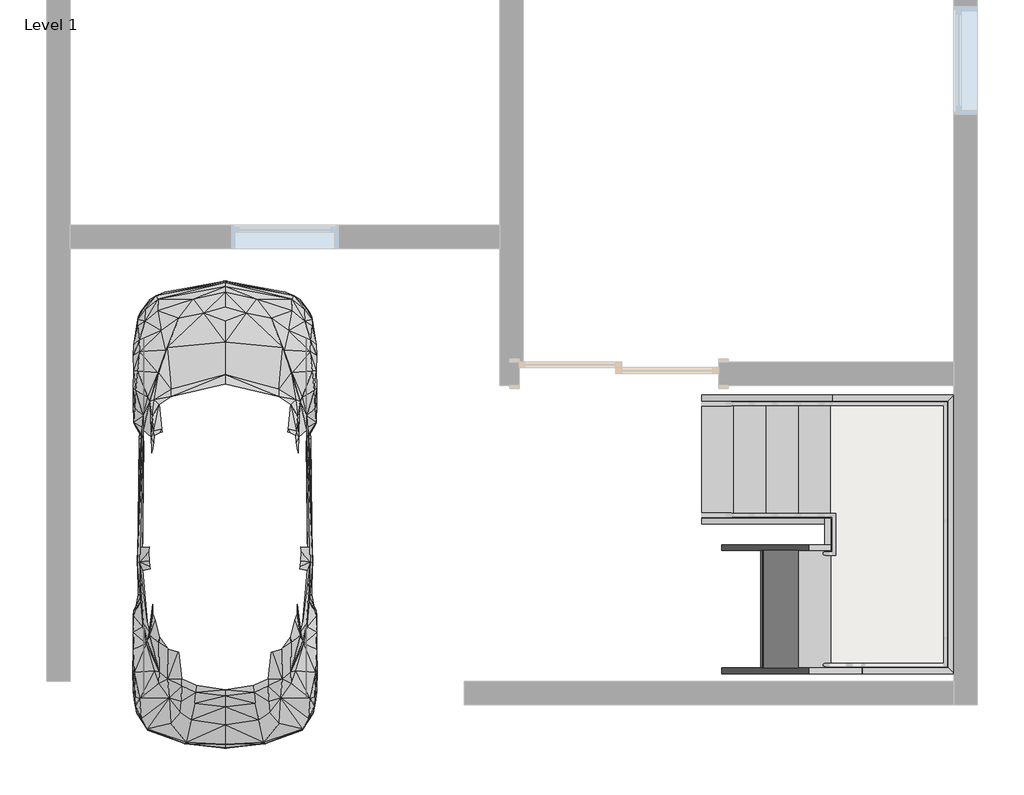
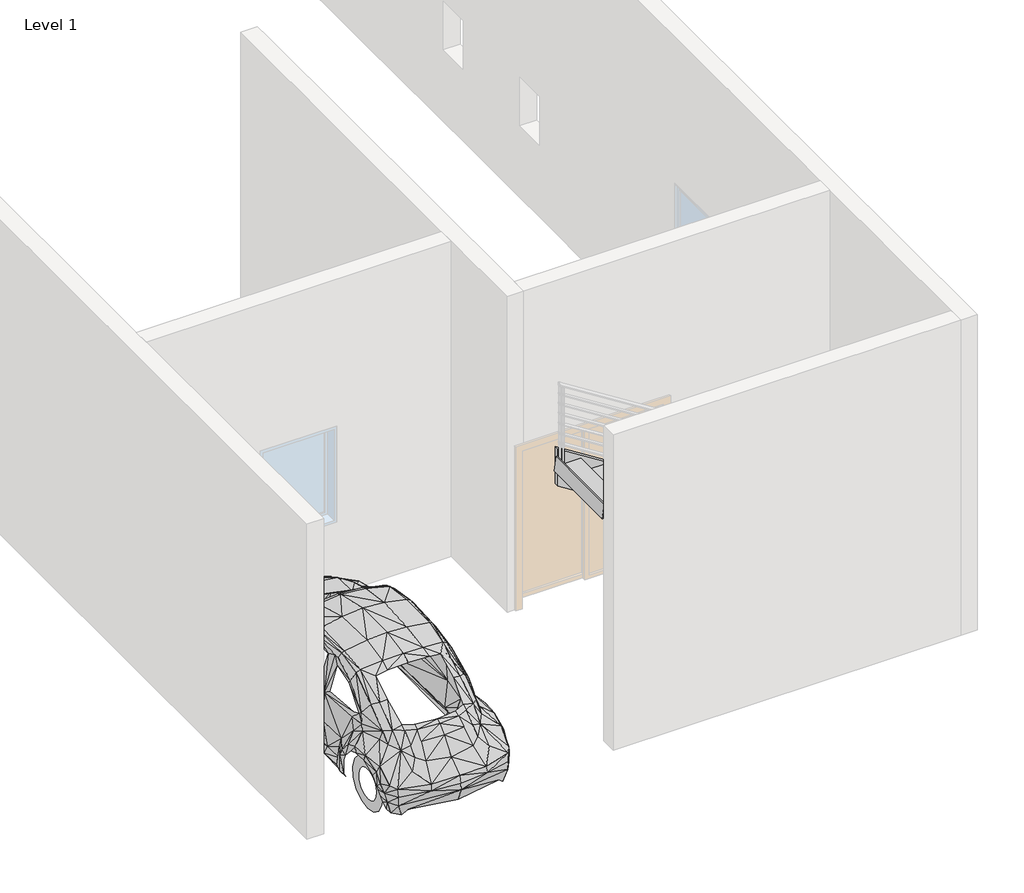
# One storey, part 4 of 4: 8 members, 2 stair flights, 1 proxy, 1 slab.
"""IFC4 building model written with IfcOpenShell, lengths in millimetres."""

from ifc_helpers import new_model, si_unit, frame, origin, place, context, project, spatial, polyline, outline, extrude, faceted_brep, transform, mapped, element, save
from components import m_rpc_beetle_m_rpc_beetle_b6d71803, non_monolithic_landing_122d3c1d, stair_flight_50mm_tread_25mm_nosing_13mm_riser_3ceddbfd, stair_flight_50mm_tread_25mm_nosing_13mm_riser_1450225a

model = new_model("IFC4")

# Units and contexts
model_context = context("Model", 3, world=origin())
ifc_project = project(units=[si_unit("LENGTHUNIT", "METRE", prefix="MILLI")], contexts=[model_context])

# Site, building, storey
site = spatial("IfcSite", under=ifc_project)
building = spatial("IfcBuilding", under=site)
storey = spatial("IfcBuildingStorey", under=building, Name="Level 1", Elevation=0.0)

# Proxy
placement = place(None, origin())
m_rpc_beetle_m_rpc_beetle_shape = m_rpc_beetle_m_rpc_beetle_b6d71803(model_context)
element("IfcBuildingElementProxy", 1, Name="M_RPC Beetle : M_RPC Beetle", ObjectType="M_RPC Beetle : M_RPC Beetle", at=placement, inside=storey, context=model_context, shape_type="MappedRepresentation", body=[
    mapped(m_rpc_beetle_m_rpc_beetle_shape, transform((-7849.5496658, -3747.5048847, 0.0), x_axis=(1.0, 0.0, 0.0), y_axis=(0.0, 1.0, 0.0), z_axis=(0.0, 0.0, 1.0))),
])

# Members
element("IfcMember", 2, ObjectType="Stringer - 50mm Width", at=placement, inside=storey, context=model_context, shape_type="SweptSolid", body=[
    extrude(outline(polyline([(215.089535, -3791.9701746), (0.0, -3791.9701746), (0.0, -3383.7114418), (516.9589444, -2566.2701111), (916.9589444, -2682.1391711), (215.089535, -3791.9701746)])), frame((0.0, -1541.1632824, 0.0), z_axis=(0.0, 1.0, 0.0), x_axis=(0.0, 0.0, 1.0)), (0.0, 0.0, 1.0), 50.0),
])
element("IfcMember", 3, ObjectType="Stringer - 50mm Width", at=placement, inside=storey, context=model_context, shape_type="SweptSolid", body=[
    extrude(outline(polyline([(215.089535, -3791.9701746), (0.0, -3791.9701746), (0.0, -3383.7114418), (405.8442796, -2741.9701746), (879.1211555, -2741.9701746), (215.089535, -3791.9701746)])), frame((0.0, -2591.1890637, 0.0), z_axis=(0.0, 1.0, 0.0), x_axis=(0.0, 0.0, 1.0)), (0.0, 0.0, 1.0), 50.0),
])
element("IfcMember", 4, ObjectType="Stringer - 50mm Width", at=placement, inside=storey, context=model_context, shape_type="SweptSolid", body=[
    extrude(outline(polyline([(516.9589444, -2542.6702382), (916.9589444, -2426.8011782), (2997.6982306, -5716.9701746), (2524.4213547, -5716.9701746), (516.9589444, -2542.6702382)])), frame((0.0, -3866.2148449, 0.0), z_axis=(0.0, 1.0, 0.0), x_axis=(0.0, 0.0, 1.0)), (0.0, 0.0, 1.0), 50.0),
])
element("IfcMember", 5, ObjectType="Stringer - 50mm Width", at=placement, inside=storey, context=model_context, shape_type="SweptSolid", body=[
    extrude(outline(polyline([(611.3778765, -2691.9701746), (1084.6547524, -2691.9701746), (2997.6982306, -5716.9701746), (2524.4213547, -5716.9701746), (611.3778765, -2691.9701746)])), frame((0.0, -2816.1890637, 0.0), z_axis=(0.0, 1.0, 0.0), x_axis=(0.0, 0.0, 1.0)), (0.0, 0.0, 1.0), 50.0),
])
element("IfcMember", 6, ObjectType="Stringer - 50mm Width", at=placement, inside=storey, context=model_context, shape_type="Brep", body=[
    faceted_brep([(-2426.8011782, -3816.2148449, 916.9589444), (-2426.8011782, -3866.2148449, 916.9589444), (-1641.9443934, -3866.2148449, 916.9589444), (-1691.9443934, -3816.2148449, 916.9589444), (-2542.6702382, -3816.2148449, 516.9589444), (-1691.9443934, -3816.2148449, 516.9589444), (-2542.6702382, -3866.2148449, 516.9589444), (-1641.9443934, -3866.2148449, 516.9589444)], [[[0, 1, 2, 3]], [[4, 0, 3, 5]], [[6, 4, 5, 7]], [[1, 6, 7, 2]], [[1, 0, 4, 6]], [[2, 7, 5, 3]]]),
])
element("IfcMember", 7, ObjectType="Stringer - 50mm Width", at=placement, inside=storey, context=model_context, shape_type="SweptSolid", body=[
    extrude(outline(polyline([(-1641.9443934, -3866.2148449), (-1691.9443934, -3816.2148449), (-1691.9443934, -1541.1632824), (-1641.9443934, -1491.1632824), (-1641.9443934, -3866.2148449)])), frame((0.0, 0.0, 516.9589444), z_axis=(0.0, 0.0, 1.0), x_axis=(1.0, 0.0, 0.0)), (0.0, 0.0, 1.0), 400.0),
])
element("IfcMember", 8, ObjectType="Stringer - 50mm Width", at=placement, inside=storey, context=model_context, shape_type="Brep", body=[
    faceted_brep([(-1691.9443934, -1541.1632824, 916.9589444), (-1641.9443934, -1491.1632824, 916.9589444), (-2682.1391711, -1491.1632824, 916.9589444), (-2682.1391711, -1541.1632824, 916.9589444), (-1691.9443934, -1541.1632824, 516.9589444), (-2566.2701111, -1541.1632824, 516.9589444), (-1641.9443934, -1491.1632824, 516.9589444), (-2566.2701111, -1491.1632824, 516.9589444)], [[[0, 1, 2, 3]], [[4, 0, 3, 5]], [[6, 4, 5, 7]], [[1, 6, 7, 2]], [[1, 0, 4, 6]], [[2, 7, 5, 3]]]),
])
element("IfcMember", 9, ObjectType="Stringer - 50mm Width", at=placement, inside=storey, context=model_context, shape_type="SweptSolid", body=[
    extrude(outline(polyline([(-2741.9701746, -2541.1890637), (-2691.9701746, -2541.1890637), (-2691.9701746, -2766.1890637), (-2741.9701746, -2766.1890637), (-2741.9701746, -2541.1890637)])), frame((0.0, 0.0, 516.9589444), z_axis=(0.0, 0.0, 1.0), x_axis=(1.0, 0.0, 0.0)), (0.0, 0.0, 1.0), 400.0),
])

# Slab
non_monolithic_landing_shape = non_monolithic_landing_122d3c1d(model_context)
element("IfcSlab", 10, ObjectType="Non-Monolithic Landing", at=placement, inside=storey, context=model_context, shape_type="MappedRepresentation", body=[
    mapped(non_monolithic_landing_shape, transform((0.0, 0.0, 0.0), x_axis=(1.0, 0.0, 0.0), y_axis=(0.0, 1.0, 0.0), z_axis=(0.0, 0.0, 1.0))),
])

# Stair flights
stair_flight_50mm_tread_25mm_nosing_13mm_riser_shape = stair_flight_50mm_tread_25mm_nosing_13mm_riser_3ceddbfd(model_context)
element("IfcStairFlight", 11, ObjectType="50mm Tread 25mm Nosing 13mm Riser", at=placement, inside=storey, context=model_context, shape_type="MappedRepresentation", body=[
    mapped(stair_flight_50mm_tread_25mm_nosing_13mm_riser_shape, transform((0.0, 0.0, 0.0), x_axis=(1.0, 0.0, 0.0), y_axis=(0.0, 1.0, 0.0), z_axis=(0.0, 0.0, 1.0))),
])
stair_flight_50mm_tread_25mm_nosing_13mm_riser_2_shape = stair_flight_50mm_tread_25mm_nosing_13mm_riser_1450225a(model_context)
element("IfcStairFlight", 12, ObjectType="50mm Tread 25mm Nosing 13mm Riser", at=placement, inside=storey, context=model_context, shape_type="MappedRepresentation", body=[
    mapped(stair_flight_50mm_tread_25mm_nosing_13mm_riser_2_shape, transform((0.0, 0.0, 0.0), x_axis=(1.0, 0.0, 0.0), y_axis=(0.0, 1.0, 0.0), z_axis=(0.0, 0.0, 1.0))),
])

save(model, "model.ifc")

# Revit data of these elements
# Type "M_RPC Beetle : M_RPC Beetle"
#   built-in parameter 1005198 = "{2, 15},{39, RPC-16-0U6E-L4EG-ENH1-J3KF-SVEL-0TX4-C0},{1, 0},{1, 0},{2, 18},{1, 8},{5, Color},{1, 0},{1, 0},{3, 0.8},{3, 0.8},{3, 0.8},{1, 8},{7, BBoxMin},{1, 0},{1, 0},{1, 0},{1, 0},{1, 0},{1, 8},{7, BBoxMax},{1, 0},{1, 0},{1, 0},{1, 0},{1, 0},{2, 11},{9, RPCTypeId},{1, 0},{1, 0},{39, RPC-16-0U6E-L4EG-ENH1-J3KF-SVEL-0TX4-C0},{1, 6},{14, RPCPlantHeight},{1, 0},{1, 0},{4, 4.92},{2, 11},{7, keyword},{1, 0},{1, 0},{39, :RPCs:Auto_Economy/Midsize:Geometry:RPC},{2, 11},{8, category},{1, 0},{1, 0},{20, Auto_Economy/Midsize},{2, 11},{12, LocalizedUID},{1, 0},{1, 0},{13, VW Beetle [4]},{2, 14},{6, Height},{1, 0},{1, 0},{4, 4.92},{1, 2},{16, Cast Reflections},{1, 0},{1, 0},{1, 0},{1, 4},{12, Transparency},{1, 0},{1, 0},{2, 18},{1, 4},{7, Tinting},{1, 0},{1, 0},{2, 50},{1, 2},{11, Use Tinting},{1, 0},{1, 0},{1, 0},{1, 2},{13, License Plate},{1, 0},{1, 0},{1, 0},{2, 11},{21, License Plate Texture},{1, 0},{1, 0},{64, __RPC:/object data/textures/car/plate/textures/default/rgb/0/0/0},{2, 11},{23, i_License Plate Texture},{1, 0},{1, 0},{0, },{1, 2},{12, Custom Plate},{1, 0},{1, 0},{1, 0},{2, 11},{23, License Plate File Name},{1, 0},{1, 0},{0, },{21, assetlibrary_base.fbx},{1, 5},"
#   built-in parameter 1005195 = "RPC-16-0U6E-L4EG-ENH1-J3KF-SVEL-0TX4-C0"
#   Height = 0
# Element 1 (IfcBuildingElementProxy, "M_RPC Beetle : M_RPC Beetle")
#   Phase Created = New Construction
# Elements 2, 3, 4, 5, 6, 7, 8, 9 (IfcMember, "Stringer - 50mm Width")
#   Phase Created = New Construction
# Element 10 (IfcSlab, "Non-Monolithic Landing")
#   Phase Created = New Construction
# Elements 11, 12 (IfcStairFlight, "50mm Tread 25mm Nosing 13mm Riser")
#   Phase Created = New Construction
